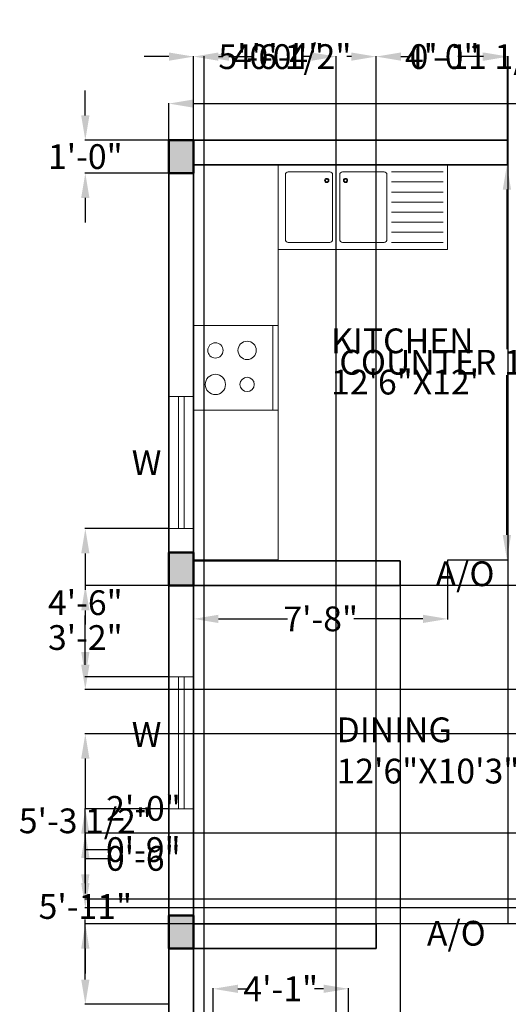
# Model space of a CAD drawing. Units: inches. Extents: x 113 to 575, y 111 to 799.
# Tile 3 of 4: x 123 to 301, y 441 to 799. Entities that reach past the tile are written whole.
import ezdxf

# ---------------------------------------------------------------- set-up
doc = ezdxf.new("R2010")
doc.units = ezdxf.units.IN
doc.header["$MEASUREMENT"] = 0
for name, color, linetype, lineweight in [('A-ANNO-DIMS', 2, 'Continuous', 18), ('A-ANNO-TEXT', 7, 'Continuous', 18), ('A-AREA-IDEN', 7, 'Continuous', 25), ('A-COLS', 7, 'Continuous', 50), ('A-COLS-PATT', 252, 'Continuous', 13), ('A-FLOR-FIXT', 9, 'Continuous', 18), ('A-GLAZ', 4, 'Continuous', 18), ('A-WALL', 7, 'Continuous', 35)]:
    doc.layers.add(name, color=color, linetype=linetype, lineweight=lineweight)
doc.styles.get("Standard").update_dxf_attribs({"font": 'arial.ttf'})
doc.dimstyles.get("Standard").update_dxf_attribs({"dimtxt": 9, "dimasz": 9, "dimexe": 0.18, "dimexo": 0.0625, "dimgap": 0.09, "dimtad": 0, "dimtih": 1, "dimtoh": 1, "dimdec": 0, "dimzin": 0, "dimdsep": 46, "dimlunit": 3, "dimtxsty": 'Standard', "dimcen": 0.09, "dimadec": 0, "dimazin": 0, "dimtfac": 1, "dimtdec": 0, "dimtofl": 0, "dimtmove": 0, "dimatfit": 3, "dimfxl": 1, "dimtolj": 1, "dimtzin": 0, "dimarcsym": 0})

# ---------------------------------------------------------------- blocks, each defined once
blk = doc.blocks.new('КУХ11 2800х1800')
for p, q in [((1200, 2801.6), (-600, 2801.6)), ((-600, 2801.6), (-600, 0)), ((0, 2201.6), (0, 2801.6)), ((1200, 2801.6), (1200, 2201.6)), ((1200, 2801.6), (1200, 2201.6)), ((50, 2271.6), (50, 2731.6)), ((70, 2751.6), (364.8, 2751.6)), ((384.8, 2731.6), (384.8, 2271.6)), ((434.8, 2731.6), (434.8, 2271.6)), ((749.6, 2751.6), (454.8, 2751.6)), ((769.6, 2271.6), (769.6, 2731.6)), ((801.4, 2751.6), (1168.2, 2751.6)), ((801.4, 2680.2), (1168.2, 2680.2)), ((801.4, 2608.8), (1168.2, 2608.8)), ((801.4, 2537.3), (1168.2, 2537.3)), ((801.4, 2465.9), (1168.2, 2465.9)), ((801.4, 2394.5), (1168.2, 2394.5)), ((801.4, 2323), (1168.2, 2323)), ((364.8, 2251.6), (70, 2251.6)), ((454.8, 2251.6), (749.6, 2251.6)), ((801.4, 2251.6), (1168.2, 2251.6)), ((0, 2201.6), (1200, 2201.6)), ((0, 0), (0, 2201.6)), ((-600, 1661.9), (0, 1661.9)), ((-39.6, 1061.9), (-39.6, 1663.5)), ((-600, 1061.9), (0, 1061.9)), ((0, 0), (-600, 0))]:
    blk.add_line(p, q)
for centre, radius in [((343.2, 2690.8), 15), ((343.2, 2690.8), 10), ((476.4, 2690.8), 15), ((476.4, 2690.8), 10), ((-446, 1485.1), 54.3), ((-221, 1485.1), 65.1), ((-446, 1243.4), 71.8), ((-221, 1243.4), 50.9)]:
    blk.add_circle(centre, radius)
for centre, start, end in [((70, 2731.6), 90, 180), ((364.8, 2731.6), 0, 90), ((454.8, 2731.6), 90, 180), ((749.6, 2731.6), 0, 90), ((70, 2271.6), 180, 270), ((364.8, 2271.6), 270, 0), ((454.8, 2271.6), 180, 270), ((749.6, 2271.6), 270, 0)]:
    blk.add_arc(centre, 20, start, end)
blk = doc.blocks.new('*D6')
at = {"layer": 'A-ANNO-DIMS', "color": 0, "lineweight": -2, "transparency": 16777216}
for p, q in [((177.49, 754.88), (177.49, 768.27)), ((186.49, 768.09), (325.69, 768.09)), ((480.49, 768.09), (341.3, 768.09)), ((489.49, 754.88), (489.49, 768.27))]:
    blk.add_line(p, q, dxfattribs=at)
at = {"layer": 'A-ANNO-DIMS', "color": 0, "transparency": 16777216}
for points in [[(186.49, 769.59), (186.49, 766.59), (177.49, 768.09)], [(480.49, 769.59), (480.49, 766.59), (489.49, 768.09)]]:
    blk.add_solid(points, dxfattribs=at)
at = {"layer": 'Defpoints', "color": 0, "transparency": 16777216}
for p in [(489.49, 768.09), (177.49, 754.81), (489.49, 754.81)]:
    blk.add_point(p, dxfattribs=at)
at = {"layer": 'A-ANNO-DIMS', "color": 0, "transparency": 16777216, "insert": (333.49, 768.09), "char_height": 9, "attachment_point": 5}
blk.add_mtext("\\A1;26'", dxfattribs=at)
blk = doc.blocks.new('WIN-48IN')
for p, q in [((0, 9), (0, 0)), ((48, 9), (48, 0)), ((0, 5.5), (48, 5.5)), ((0, 3.5), (48, 3.5))]:
    blk.add_line(p, q)
blk = doc.blocks.new('*D18')
at = {"layer": 'A-ANNO-DIMS', "color": 0, "lineweight": -2, "transparency": 16777216}
for p, q in [((278.8, 745.81), (300.45, 745.81)), ((300.27, 736.81), (300.27, 678.78)), ((300.27, 611.24), (300.27, 669.28)), ((278.8, 602.24), (300.45, 602.24))]:
    blk.add_line(p, q, dxfattribs=at)
at = {"layer": 'A-ANNO-DIMS', "color": 0, "transparency": 16777216}
for points in [[(298.77, 736.81), (301.77, 736.81), (300.27, 745.81)], [(298.77, 611.24), (301.77, 611.24), (300.27, 602.24)]]:
    blk.add_solid(points, dxfattribs=at)
at = {"layer": 'Defpoints', "color": 0, "transparency": 16777216}
for p in [(278.74, 745.81), (300.27, 745.81), (278.74, 602.24)]:
    blk.add_point(p, dxfattribs=at)
at = {"layer": 'A-ANNO-DIMS', "color": 0, "transparency": 16777216, "insert": (300.27, 674.03), "char_height": 9, "attachment_point": 5}
blk.add_mtext('\\A1;COUNTER 11\'-11 1/2"', dxfattribs=at)
blk = doc.blocks.new('*D19')
at = {"layer": 'A-ANNO-DIMS', "color": 0, "lineweight": -2, "transparency": 16777216}
for p, q in [((186.49, 602.18), (186.49, 580.53)), ((278.74, 602.18), (278.74, 580.53)), ((195.49, 580.71), (220.6, 580.71)), ((269.74, 580.71), (244.63, 580.71))]:
    blk.add_line(p, q, dxfattribs=at)
at = {"layer": 'A-ANNO-DIMS', "color": 0, "transparency": 16777216}
for points in [[(195.49, 582.21), (195.49, 579.21), (186.49, 580.71)], [(269.74, 582.21), (269.74, 579.21), (278.74, 580.71)]]:
    blk.add_solid(points, dxfattribs=at)
at = {"layer": 'Defpoints', "color": 0, "transparency": 16777216}
for p in [(186.49, 602.24), (278.74, 602.24), (278.74, 580.71)]:
    blk.add_point(p, dxfattribs=at)
at = {"layer": 'A-ANNO-DIMS', "color": 0, "transparency": 16777216, "insert": (232.62, 580.71), "char_height": 9, "attachment_point": 5}
blk.add_mtext('\\A1;7\'-8"', dxfattribs=at)
blk = doc.blocks.new('*D21')
at = {"layer": 'A-ANNO-DIMS', "color": 0, "lineweight": -2, "transparency": 16777216}
for p, q in [((193.54, 435.74), (193.54, 446.38)), ((202.54, 446.2), (205.88, 446.2)), ((233.68, 446.2), (230.35, 446.2)), ((242.68, 435.74), (242.68, 446.38))]:
    blk.add_line(p, q, dxfattribs=at)
at = {"layer": 'A-ANNO-DIMS', "color": 0, "transparency": 16777216}
for points in [[(202.54, 447.7), (202.54, 444.7), (193.54, 446.2)], [(233.68, 447.7), (233.68, 444.7), (242.68, 446.2)]]:
    blk.add_solid(points, dxfattribs=at)
at = {"layer": 'Defpoints', "color": 0, "transparency": 16777216}
for p in [(193.54, 446.2), (193.54, 435.68), (242.68, 435.68)]:
    blk.add_point(p, dxfattribs=at)
at = {"layer": 'A-ANNO-DIMS', "color": 0, "transparency": 16777216, "insert": (218.11, 446.2), "char_height": 9, "attachment_point": 5}
blk.add_mtext('\\A1;4\'-1"', dxfattribs=at)
blk = doc.blocks.new('*D28')
at = {"layer": 'A-ANNO-DIMS', "color": 0, "lineweight": -2, "transparency": 16777216}
for p, q in [((190.28, 250.88), (190.28, 785.35)), ((199.28, 785.17), (202.05, 785.17)), ((229.28, 785.17), (226.51, 785.17)), ((238.28, 250.88), (238.28, 785.35))]:
    blk.add_line(p, q, dxfattribs=at)
at = {"layer": 'A-ANNO-DIMS', "color": 0, "transparency": 16777216}
for points in [[(199.28, 786.67), (199.28, 783.67), (190.28, 785.17)], [(229.28, 786.67), (229.28, 783.67), (238.28, 785.17)]]:
    blk.add_solid(points, dxfattribs=at)
at = {"layer": 'Defpoints', "color": 0, "transparency": 16777216}
for p in [(238.28, 785.17), (190.28, 250.81), (238.28, 250.81)]:
    blk.add_point(p, dxfattribs=at)
at = {"layer": 'A-ANNO-DIMS', "color": 0, "transparency": 16777216, "insert": (214.28, 785.17), "char_height": 9, "attachment_point": 5}
blk.add_mtext('\\A1;4\'-0"', dxfattribs=at)
blk = doc.blocks.new('*D29')
at = {"layer": 'A-ANNO-DIMS', "color": 0, "lineweight": -2, "transparency": 16777216}
for p, q in [((291.494828, 785.172567), (282.494828, 785.172567)), ((300.494828, 754.875317), (300.494828, 785.352567)), ((336.494828, 754.875317), (336.494828, 785.352567)), ((345.494828, 785.172567), (354.494828, 785.172567))]:
    blk.add_line(p, q, dxfattribs=at)
at = {"layer": 'A-ANNO-DIMS', "color": 0, "transparency": 16777216}
for points in [[(291.494828, 786.672567), (291.494828, 783.672567), (300.494828, 785.172567)], [(345.494828, 786.672567), (345.494828, 783.672567), (336.494828, 785.172567)]]:
    blk.add_solid(points, dxfattribs=at)
at = {"layer": 'Defpoints', "color": 0, "transparency": 16777216}
for p in [(336.494828, 785.172567), (300.494828, 754.812817), (336.494828, 754.812817)]:
    blk.add_point(p, dxfattribs=at)
at = {"layer": 'A-ANNO-DIMS', "color": 0, "transparency": 16777216, "insert": (318.494828, 785.172567), "char_height": 9, "attachment_point": 5}
blk.add_mtext('\\A1;3\'-0"', dxfattribs=at)
blk = doc.blocks.new('*D30')
at = {"layer": 'A-ANNO-DIMS', "color": 0, "lineweight": -2, "transparency": 16777216}
for p, q in [((252.77, 469.88), (252.77, 785.35)), ((261.77, 785.17), (264.53, 785.17)), ((291.77, 785.17), (289, 785.17)), ((300.77, 469.88), (300.77, 785.35))]:
    blk.add_line(p, q, dxfattribs=at)
at = {"layer": 'A-ANNO-DIMS', "color": 0, "transparency": 16777216}
for points in [[(261.77, 786.67), (261.77, 783.67), (252.77, 785.17)], [(291.77, 786.67), (291.77, 783.67), (300.77, 785.17)]]:
    blk.add_solid(points, dxfattribs=at)
at = {"layer": 'Defpoints', "color": 0, "transparency": 16777216}
for p in [(300.77, 785.17), (252.77, 469.81), (300.77, 469.81)]:
    blk.add_point(p, dxfattribs=at)
at = {"layer": 'A-ANNO-DIMS', "color": 0, "transparency": 16777216, "insert": (276.77, 785.17), "char_height": 9, "attachment_point": 5}
blk.add_mtext('\\A1;4\'-0"', dxfattribs=at)
blk = doc.blocks.new('*D31')
at = {"layer": 'A-ANNO-DIMS', "color": 0, "lineweight": -2, "transparency": 16777216}
for p, q in [((147.14, 502.81), (147.14, 511.81)), ((147.14, 511.81), (156.14, 511.81)), ((416.43, 502.81), (146.96, 502.81)), ((147.14, 487.81), (147.14, 493.81)), ((416.43, 478.81), (146.96, 478.81))]:
    blk.add_line(p, q, dxfattribs=at)
at = {"layer": 'A-ANNO-DIMS', "color": 0, "transparency": 16777216}
for points in [[(145.64, 493.81), (148.64, 493.81), (147.14, 502.81)], [(145.64, 487.81), (148.64, 487.81), (147.14, 478.81)]]:
    blk.add_solid(points, dxfattribs=at)
at = {"layer": 'Defpoints', "color": 0, "transparency": 16777216}
for p in [(147.14, 502.81), (416.49, 502.81), (416.49, 478.81)]:
    blk.add_point(p, dxfattribs=at)
at = {"layer": 'A-ANNO-DIMS', "color": 0, "transparency": 16777216, "insert": (168.26, 511.81), "char_height": 9, "attachment_point": 5}
blk.add_mtext('\\A1;2\'-0"', dxfattribs=at)
blk = doc.blocks.new('*D36')
at = {"layer": 'A-ANNO-DIMS', "color": 0, "lineweight": -2, "transparency": 16777216}
for p, q in [((177.43, 511.67), (146.96, 511.67)), ((147.14, 502.67), (147.14, 480.8)), ((147.14, 449.56), (147.14, 471.43)), ((177.43, 440.56), (146.96, 440.56))]:
    blk.add_line(p, q, dxfattribs=at)
at = {"layer": 'A-ANNO-DIMS', "color": 0, "transparency": 16777216}
for points in [[(145.64, 502.67), (148.64, 502.67), (147.14, 511.67)], [(145.64, 449.56), (148.64, 449.56), (147.14, 440.56)]]:
    blk.add_solid(points, dxfattribs=at)
at = {"layer": 'Defpoints', "color": 0, "transparency": 16777216}
for p in [(147.14, 511.67), (177.49, 511.67), (177.49, 440.56)]:
    blk.add_point(p, dxfattribs=at)
at = {"layer": 'A-ANNO-DIMS', "color": 0, "transparency": 16777216, "insert": (147.14, 476.12), "char_height": 9, "attachment_point": 5}
blk.add_mtext('\\A1;5\'-11"', dxfattribs=at)
blk = doc.blocks.new('*D37')
at = {"layer": 'A-ANNO-DIMS', "color": 0, "lineweight": -2, "transparency": 16777216}
for p, q in [((177.43, 613.52), (146.96, 613.52)), ((147.14, 604.52), (147.14, 591.28)), ((147.14, 568.67), (147.14, 581.91)), ((177.43, 559.67), (146.96, 559.67))]:
    blk.add_line(p, q, dxfattribs=at)
at = {"layer": 'A-ANNO-DIMS', "color": 0, "transparency": 16777216}
for points in [[(145.64, 604.52), (148.64, 604.52), (147.14, 613.52)], [(145.64, 568.67), (148.64, 568.67), (147.14, 559.67)]]:
    blk.add_solid(points, dxfattribs=at)
at = {"layer": 'Defpoints', "color": 0, "transparency": 16777216}
for p in [(147.14, 613.52), (177.49, 613.52), (177.49, 559.67)]:
    blk.add_point(p, dxfattribs=at)
at = {"layer": 'A-ANNO-DIMS', "color": 0, "transparency": 16777216, "insert": (147.14, 586.6), "char_height": 9, "attachment_point": 5}
blk.add_mtext('\\A1;4\'-6"', dxfattribs=at)
blk = doc.blocks.new('*D42')
at = {"layer": 'A-ANNO-DIMS', "color": 0, "lineweight": -2, "transparency": 16777216}
for p, q in [((327.49, 785.17), (318.49, 785.17)), ((336.49, 754.88), (336.49, 785.35)), ((348.21, 754.88), (348.21, 785.35)), ((357.21, 785.17), (366.21, 785.17))]:
    blk.add_line(p, q, dxfattribs=at)
at = {"layer": 'A-ANNO-DIMS', "color": 0, "transparency": 16777216}
for points in [[(327.49, 786.67), (327.49, 783.67), (336.49, 785.17)], [(357.21, 786.67), (357.21, 783.67), (348.21, 785.17)]]:
    blk.add_solid(points, dxfattribs=at)
at = {"layer": 'Defpoints', "color": 0, "transparency": 16777216}
for p in [(336.49, 785.17), (336.49, 754.81), (348.21, 754.81)]:
    blk.add_point(p, dxfattribs=at)
at = {"layer": 'A-ANNO-DIMS', "color": 0, "transparency": 16777216, "insert": (292.46, 785.17), "char_height": 9, "attachment_point": 5}
blk.add_mtext('\\A1;0\'-11 1/2"', dxfattribs=at)
blk = doc.blocks.new('*D45')
at = {"layer": 'A-ANNO-DIMS', "color": 0, "lineweight": -2, "transparency": 16777216}
for p, q in [((336.43, 592.81), (146.96, 592.81)), ((147.14, 583.81), (147.14, 578.61)), ((147.14, 564.04), (147.14, 569.24)), ((336.43, 555.04), (146.96, 555.04))]:
    blk.add_line(p, q, dxfattribs=at)
at = {"layer": 'A-ANNO-DIMS', "color": 0, "transparency": 16777216}
for points in [[(145.64, 583.81), (148.64, 583.81), (147.14, 592.81)], [(145.64, 564.04), (148.64, 564.04), (147.14, 555.04)]]:
    blk.add_solid(points, dxfattribs=at)
at = {"layer": 'Defpoints', "color": 0, "transparency": 16777216}
for p in [(147.14, 592.81), (336.49, 592.81), (336.49, 555.04)]:
    blk.add_point(p, dxfattribs=at)
at = {"layer": 'A-ANNO-DIMS', "color": 0, "transparency": 16777216, "insert": (147.14, 573.93), "char_height": 9, "attachment_point": 5}
blk.add_mtext('\\A1;3\'-2"', dxfattribs=at)
blk = doc.blocks.new('*D46')
at = {"layer": 'A-ANNO-DIMS', "color": 0, "lineweight": -2, "transparency": 16777216}
for p, q in [((336.43, 538.91), (146.96, 538.91)), ((147.14, 529.91), (147.14, 512.01)), ((147.14, 484.62), (147.14, 502.52)), ((336.43, 475.62), (146.96, 475.62))]:
    blk.add_line(p, q, dxfattribs=at)
at = {"layer": 'A-ANNO-DIMS', "color": 0, "transparency": 16777216}
for points in [[(145.64, 529.91), (148.64, 529.91), (147.14, 538.91)], [(145.64, 484.62), (148.64, 484.62), (147.14, 475.62)]]:
    blk.add_solid(points, dxfattribs=at)
at = {"layer": 'Defpoints', "color": 0, "transparency": 16777216}
for p in [(147.14, 538.91), (336.49, 538.91), (336.49, 475.62)]:
    blk.add_point(p, dxfattribs=at)
at = {"layer": 'A-ANNO-DIMS', "color": 0, "transparency": 16777216, "insert": (147.14, 507.27), "char_height": 9, "attachment_point": 5}
blk.add_mtext('\\A1;5\'-3 1/2"', dxfattribs=at)
blk = doc.blocks.new('*D48')
at = {"layer": 'A-ANNO-DIMS', "color": 0, "lineweight": -2, "transparency": 16777216}
for p, q in [((186.49, 592.75), (186.49, 124.27)), ((261.49, 592.75), (261.49, 124.27)), ((195.49, 124.45), (211.92, 124.45)), ((252.49, 124.45), (236.07, 124.45))]:
    blk.add_line(p, q, dxfattribs=at)
at = {"layer": 'A-ANNO-DIMS', "color": 0, "transparency": 16777216}
for points in [[(195.49, 125.95), (195.49, 122.95), (186.49, 124.45)], [(252.49, 125.95), (252.49, 122.95), (261.49, 124.45)]]:
    blk.add_solid(points, dxfattribs=at)
at = {"layer": 'Defpoints', "color": 0, "transparency": 16777216}
for p in [(186.49, 592.81), (261.49, 592.81), (261.49, 124.45)]:
    blk.add_point(p, dxfattribs=at)
at = {"layer": 'A-ANNO-DIMS', "color": 0, "transparency": 16777216, "insert": (223.99, 124.45), "char_height": 9, "attachment_point": 5}
blk.add_mtext('\\A1;6\'-3"', dxfattribs=at)
blk = doc.blocks.new('*D49')
at = {"layer": 'A-ANNO-DIMS', "color": 0, "lineweight": -2, "transparency": 16777216}
for p, q in [((309.494828, 592.750317), (309.494828, 124.273067)), ((336.494828, 592.750317), (336.494828, 124.273067)), ((300.494828, 124.453067), (291.494828, 124.453067)), ((345.494828, 124.453067), (354.494828, 124.453067))]:
    blk.add_line(p, q, dxfattribs=at)
at = {"layer": 'A-ANNO-DIMS', "color": 0, "transparency": 16777216}
for points in [[(300.494828, 125.953067), (300.494828, 122.953067), (309.494828, 124.453067)], [(345.494828, 125.953067), (345.494828, 122.953067), (336.494828, 124.453067)]]:
    blk.add_solid(points, dxfattribs=at)
at = {"layer": 'Defpoints', "color": 0, "transparency": 16777216}
for p in [(309.494828, 592.812817), (336.494828, 592.812817), (336.494828, 124.453067)]:
    blk.add_point(p, dxfattribs=at)
at = {"layer": 'A-ANNO-DIMS', "color": 0, "transparency": 16777216, "insert": (322.994828, 124.453067), "char_height": 9, "attachment_point": 5}
blk.add_mtext('\\A1;2\'-3"', dxfattribs=at)
blk = doc.blocks.new('*D50')
at = {"layer": 'A-ANNO-DIMS', "color": 0, "lineweight": -2, "transparency": 16777216}
for p, q in [((186.49, 469.88), (186.49, 785.35)), ((195.49, 785.17), (197.09, 785.17)), ((243.77, 785.17), (242.17, 785.17)), ((252.77, 469.88), (252.77, 785.35))]:
    blk.add_line(p, q, dxfattribs=at)
at = {"layer": 'A-ANNO-DIMS', "color": 0, "transparency": 16777216}
for points in [[(195.49, 786.67), (195.49, 783.67), (186.49, 785.17)], [(243.77, 786.67), (243.77, 783.67), (252.77, 785.17)]]:
    blk.add_solid(points, dxfattribs=at)
at = {"layer": 'Defpoints', "color": 0, "transparency": 16777216}
for p in [(252.77, 785.17), (186.49, 469.81), (252.77, 469.81)]:
    blk.add_point(p, dxfattribs=at)
at = {"layer": 'A-ANNO-DIMS', "color": 0, "transparency": 16777216, "insert": (219.63, 785.17), "char_height": 9, "attachment_point": 5}
blk.add_mtext('\\A1;5\'-6 1/2"', dxfattribs=at)
blk = doc.blocks.new('*D51')
at = {"layer": 'A-ANNO-DIMS', "color": 0, "lineweight": -2, "transparency": 16777216}
for p, q in [((147.135078, 763.812817), (147.135078, 772.812817)), ((177.432328, 754.812817), (146.955078, 754.812817)), ((177.432328, 742.812817), (146.955078, 742.812817)), ((147.135078, 733.812817), (147.135078, 724.812817))]:
    blk.add_line(p, q, dxfattribs=at)
at = {"layer": 'A-ANNO-DIMS', "color": 0, "transparency": 16777216}
for points in [[(145.635078, 763.812817), (148.635078, 763.812817), (147.135078, 754.812817)], [(145.635078, 733.812817), (148.635078, 733.812817), (147.135078, 742.812817)]]:
    blk.add_solid(points, dxfattribs=at)
at = {"layer": 'Defpoints', "color": 0, "transparency": 16777216}
for p in [(177.494828, 754.812817), (147.135078, 742.812817), (177.494828, 742.812817)]:
    blk.add_point(p, dxfattribs=at)
at = {"layer": 'A-ANNO-DIMS', "color": 0, "transparency": 16777216, "insert": (147.135078, 748.812817), "char_height": 9, "attachment_point": 5}
blk.add_mtext('\\A1;1\'-0"', dxfattribs=at)
blk = doc.blocks.new('*D53')
at = {"layer": 'A-ANNO-DIMS', "color": 0, "lineweight": -2, "transparency": 16777216}
for p, q in [((177.49, 785.17), (168.49, 785.17)), ((186.49, 250.88), (186.49, 785.35)), ((190.28, 250.88), (190.28, 785.35)), ((199.28, 785.17), (208.28, 785.17))]:
    blk.add_line(p, q, dxfattribs=at)
at = {"layer": 'A-ANNO-DIMS', "color": 0, "transparency": 16777216}
for points in [[(177.49, 786.67), (177.49, 783.67), (186.49, 785.17)], [(199.28, 786.67), (199.28, 783.67), (190.28, 785.17)]]:
    blk.add_solid(points, dxfattribs=at)
at = {"layer": 'Defpoints', "color": 0, "transparency": 16777216}
for p in [(190.28, 785.17), (186.49, 250.81), (190.28, 250.81)]:
    blk.add_point(p, dxfattribs=at)
at = {"layer": 'A-ANNO-DIMS', "color": 0, "transparency": 16777216, "insert": (220.33, 785.17), "char_height": 9, "attachment_point": 5}
blk.add_mtext('\\A1;0\'-4"', dxfattribs=at)
blk = doc.blocks.new('*D54')
at = {"layer": 'A-ANNO-DIMS', "color": 0, "lineweight": -2, "transparency": 16777216}
for p, q in [((147.14, 487.81), (147.14, 496.81)), ((147.14, 496.81), (156.14, 496.81)), ((416.43, 478.81), (146.96, 478.81)), ((416.43, 469.81), (146.96, 469.81)), ((147.14, 460.81), (147.14, 451.81))]:
    blk.add_line(p, q, dxfattribs=at)
at = {"layer": 'A-ANNO-DIMS', "color": 0, "transparency": 16777216}
for points in [[(145.64, 487.81), (148.64, 487.81), (147.14, 478.81)], [(145.64, 460.81), (148.64, 460.81), (147.14, 469.81)]]:
    blk.add_solid(points, dxfattribs=at)
at = {"layer": 'Defpoints', "color": 0, "transparency": 16777216}
for p in [(147.14, 478.81), (416.49, 478.81), (416.49, 469.81)]:
    blk.add_point(p, dxfattribs=at)
at = {"layer": 'A-ANNO-DIMS', "color": 0, "transparency": 16777216, "insert": (168.19, 496.81), "char_height": 9, "attachment_point": 5}
blk.add_mtext('\\A1;0\'-9"', dxfattribs=at)
blk = doc.blocks.new('*D56')
at = {"layer": 'A-ANNO-DIMS', "color": 0, "lineweight": -2, "transparency": 16777216}
for p, q in [((147.14, 484.62), (147.14, 493.62)), ((147.14, 493.62), (156.14, 493.62)), ((336.43, 475.62), (146.96, 475.62)), ((336.43, 469.81), (146.96, 469.81)), ((147.14, 460.81), (147.14, 451.81))]:
    blk.add_line(p, q, dxfattribs=at)
at = {"layer": 'A-ANNO-DIMS', "color": 0, "transparency": 16777216}
for points in [[(145.64, 484.62), (148.64, 484.62), (147.14, 475.62)], [(145.64, 460.81), (148.64, 460.81), (147.14, 469.81)]]:
    blk.add_solid(points, dxfattribs=at)
at = {"layer": 'Defpoints', "color": 0, "transparency": 16777216}
for p in [(147.14, 475.62), (336.49, 475.62), (336.49, 469.81)]:
    blk.add_point(p, dxfattribs=at)
at = {"layer": 'A-ANNO-DIMS', "color": 0, "transparency": 16777216, "insert": (168.19, 493.62), "char_height": 9, "attachment_point": 5}
blk.add_mtext('\\A1;0\'-6"', dxfattribs=at)

msp = doc.modelspace()

# ---------------------------------------------------------------- hatches: boundary and pattern name
at = {"layer": 'A-COLS-PATT'}
h = msp.add_hatch(color=256, dxfattribs=at)
h.dxf.hatch_style = 1
h.paths.add_polyline_path([(186.49, 754.81), (177.49, 754.81), (177.49, 742.81), (186.49, 742.81)])
h.paths.add_polyline_path([(345.49, 754.81), (336.49, 754.81), (336.49, 742.81), (345.49, 742.81)])
h.paths.add_polyline_path([(489.49, 754.81), (480.49, 754.81), (480.49, 742.81), (489.49, 742.81)])
h.paths.add_polyline_path([(489.49, 601.81), (480.49, 601.81), (480.49, 589.81), (489.49, 589.81)])
h.paths.add_polyline_path([(345.49, 604.81), (336.49, 604.81), (336.49, 592.81), (345.49, 592.81)])
h.paths.add_polyline_path([(186.49, 604.81), (177.49, 604.81), (177.49, 592.81), (186.49, 592.81)])
h.paths.add_polyline_path([(186.49, 472.81), (177.49, 472.81), (177.49, 460.81), (186.49, 460.81)])
h.paths.add_polyline_path([(345.49, 469.81), (336.49, 469.81), (336.49, 457.81), (345.49, 457.81)])
h.paths.add_polyline_path([(489.49, 469.81), (480.49, 469.81), (480.49, 457.81), (489.49, 457.81)])
h.paths.add_polyline_path([(186.49, 253.81), (177.49, 253.81), (177.49, 241.81), (186.49, 241.81)])
h.paths.add_polyline_path([(345.49, 253.81), (336.49, 253.81), (336.49, 241.81), (345.49, 241.81)])
h.paths.add_polyline_path([(489.49, 253.81), (480.49, 253.81), (480.49, 241.81), (489.49, 241.81)])
h.paths.add_polyline_path([(489.49, 163.81), (477.49, 163.81), (477.49, 154.81), (489.49, 154.81)])
h.paths.add_polyline_path([(348.49, 163.81), (336.49, 163.81), (336.49, 154.81), (348.49, 154.81)])
h.paths.add_polyline_path([(189.49, 163.81), (177.49, 163.81), (177.49, 154.81), (189.49, 154.81)])

# ---------------------------------------------------------------- linework, layer by layer
at = {"layer": 'A-COLS'}
for points in [[(177.49, 754.81), (186.49, 754.81), (186.49, 742.81), (177.49, 742.81)], [(177.49, 604.81), (186.49, 604.81), (186.49, 592.81), (177.49, 592.81)], [(177.49, 472.81), (186.49, 472.81), (186.49, 460.81), (177.49, 460.81)]]:
    msp.add_lwpolyline(points, close=True, dxfattribs=at)
at = {"layer": 'A-WALL'}
for p, q in [((177.49, 754.81), (300.49, 754.81)), ((177.49, 154.81), (177.49, 754.81)), ((300.49, 754.81), (300.49, 745.81)), ((186.49, 745.81), (300.49, 745.81)), ((186.49, 601.81), (186.49, 745.81)), ((186.49, 601.81), (261.49, 601.81)), ((261.49, 601.81), (261.49, 592.81)), ((186.49, 163.81), (186.49, 592.81)), ((186.49, 592.81), (261.49, 592.81)), ((186.49, 469.81), (252.77, 469.81)), ((252.77, 469.81), (252.77, 460.81)), ((186.49, 460.81), (252.77, 460.81))]:
    msp.add_line(p, q, dxfattribs=at)

# ---------------------------------------------------------------- block references
at = {"layer": 'A-FLOR-FIXT', "xscale": 0.0512449767258657, "yscale": 0.0512449767258657, "zscale": 0.0512449767258657}
msp.add_blockref('КУХ11 2800х1800', (217.24, 602.24), dxfattribs=at)
at = {"layer": 'A-GLAZ'}
for p, rotation in [((186.49, 613.52), 90.00000000000011), ((186.49, 511.67), 90.00000000000006)]:
    msp.add_blockref('WIN-48IN', p, dxfattribs=dict(at, rotation=rotation))

# ---------------------------------------------------------------- texts
at = {"layer": 'A-ANNO-TEXT', "char_height": 9, "attachment_point": 1}
for s, insert in [('W', (164, 642.01)), ('A/O', (274.37, 601.62)), ('W', (164, 543.16)), ('A/O', (271.2, 470.9))]:
    msp.add_mtext_dynamic_manual_height_columns(s, width=17.4228, gutter_width=1, heights=[0], dxfattribs=dict(at, insert=insert))
at = {"layer": 'A-AREA-IDEN', "char_height": 9, "attachment_point": 1}
for s, insert in [('KITCHEN\\P12\'6"X12\'', (236.39, 686.31)), ('DINING\\P12\'6"X10\'3"', (238.38, 544.87))]:
    msp.add_mtext_dynamic_manual_height_columns(s, width=130.397, gutter_width=1, heights=[0], dxfattribs=dict(at, insert=insert))

# ---------------------------------------------------------------- dimensions: what is measured, and where the dimension line sits
at = {"layer": 'A-ANNO-DIMS'}
for base, p1, p2, override, picture, middle in [((252.77, 785.17), (186.49, 469.81), (252.77, 469.81), {"dimdec": 1, "dimlfac": 1, "dimrnd": 0, "dimzin": 1, "dimdsep": 46, "dimlunit": 4, "dimfrac": 2}, '*D50', (219.63, 785.17)), ((336.49, 785.17), (348.21, 754.81), (336.49, 754.81), {"dimdec": 1, "dimlfac": 1, "dimrnd": 0, "dimzin": 1, "dimdsep": 46, "dimlunit": 4, "dimfrac": 2}, '*D42', (292.46, 785.17)), ((190.28, 785.17), (186.49, 250.81), (190.28, 250.81), {"dimdec": 1, "dimlfac": 1, "dimrnd": 0, "dimzin": 1, "dimdsep": 46, "dimlunit": 4, "dimfrac": 2}, '*D53', (220.33, 785.17)), ((238.28, 785.17), (190.28, 250.81), (238.28, 250.81), {"dimdec": 1, "dimlfac": 1, "dimrnd": 0, "dimzin": 1, "dimdsep": 46, "dimlunit": 4, "dimfrac": 2}, '*D28', (214.28, 785.17)), ((300.77, 785.17), (252.77, 469.81), (300.77, 469.81), {"dimdec": 1, "dimlfac": 1, "dimrnd": 0, "dimzin": 1, "dimdsep": 46, "dimlunit": 4, "dimfrac": 2}, '*D30', (276.77, 785.17)), ((336.49, 785.17), (300.49, 754.81), (336.49, 754.81), {"dimdec": 1, "dimlfac": 1, "dimrnd": 0, "dimzin": 1, "dimdsep": 46, "dimlunit": 4, "dimfrac": 2}, '*D29', (318.49, 785.17)), ((489.49, 768.09), (177.49, 754.81), (489.49, 754.81), {"dimclrd": 0, "dimclre": 0, "dimclrt": 0}, '*D6', (333.49, 768.09)), ((278.7358, 580.7091), (186.4948, 602.2444), (278.7358, 602.2444), {"dimdec": 1, "dimlfac": 1, "dimrnd": 0, "dimzin": 1, "dimdsep": 46, "dimlunit": 4, "dimfrac": 2}, '*D19', (232.6153, 580.7091)), ((261.49, 124.45), (186.49, 592.81), (261.49, 592.81), {"dimdec": 1, "dimlfac": 1, "dimrnd": 0, "dimzin": 1, "dimdsep": 46, "dimlunit": 4, "dimfrac": 2}, '*D48', (223.99, 124.45)), ((336.49, 124.45), (309.49, 592.81), (336.49, 592.81), {"dimdec": 1, "dimlfac": 1, "dimrnd": 0, "dimzin": 1, "dimdsep": 46, "dimlunit": 4, "dimfrac": 2}, '*D49', (322.99, 124.45))]:
    dim = msp.add_linear_dim(base=base, p1=p1, p2=p2, dimstyle='Standard', override=override, dxfattribs=at)
    dim.commit()
    dim.dimension.update_dxf_attribs({"geometry": picture, "text_midpoint": middle})
for base, p1, p2, angle, picture, middle in [((147.14, 742.81), (177.49, 754.81), (177.49, 742.81), 90, '*D51', (147.14, 748.81)), ((147.1351, 613.5238), (177.4948, 559.6729), (177.4948, 613.5238), 90, '*D37', (147.1351, 586.5983)), ((147.14, 592.81), (336.49, 555.04), (336.49, 592.81), 90, '*D45', (147.14, 573.93)), ((147.14, 538.91), (336.49, 475.62), (336.49, 538.91), 90, '*D46', (147.14, 507.27)), ((147.14, 502.81), (416.49, 478.81), (416.49, 502.81), 90, '*D31', (168.26, 511.81)), ((147.14, 511.67), (177.49, 440.56), (177.49, 511.67), 90, '*D36', (147.14, 476.12)), ((147.14, 478.81), (416.49, 469.81), (416.49, 478.81), 90, '*D54', (168.19, 496.81)), ((147.14, 475.62), (336.49, 469.81), (336.49, 475.62), 90, '*D56', (168.19, 493.62)), ((193.54, 446.2), (242.68, 435.68), (193.54, 435.68), 180, '*D21', (218.11, 446.2))]:
    dim = msp.add_linear_dim(base=base, p1=p1, p2=p2, angle=angle, dimstyle='Standard', override={"dimdec": 1, "dimlfac": 1, "dimrnd": 0, "dimzin": 1, "dimdsep": 46, "dimlunit": 4, "dimfrac": 2}, dxfattribs=at)
    dim.commit()
    dim.dimension.update_dxf_attribs({"geometry": picture, "text_midpoint": middle})
dim = msp.add_linear_dim(base=(300.27, 745.81), p1=(278.74, 602.24), p2=(278.74, 745.81), angle=90, text='COUNTER <>', dimstyle='Standard', override={"dimdec": 1, "dimlfac": 1, "dimrnd": 0, "dimzin": 1, "dimdsep": 46, "dimlunit": 4, "dimfrac": 2}, dxfattribs=at)
dim.commit()
dim.dimension.update_dxf_attribs({"geometry": '*D18', "text_midpoint": (300.27, 674.03)})

doc.saveas('drawing.dxf')
